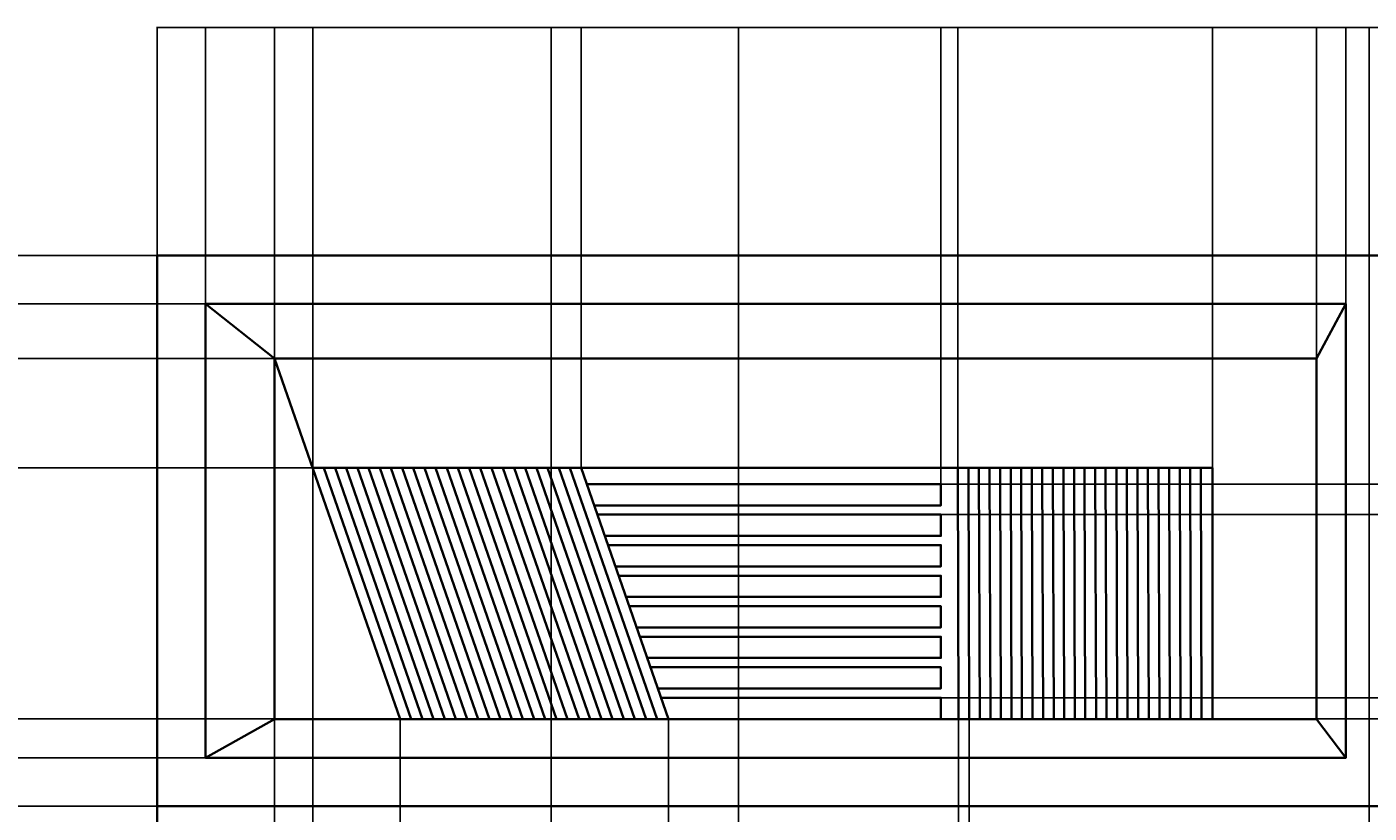
# Model space of a CAD drawing. Units: feet. Extents: x 1141 to 2858, y 751 to 1654.
# Tile 12 of 13: x 2288 to 2610, y 1466 to 1654. Entities that reach past the tile are written whole.
import ezdxf

# ---------------------------------------------------------------- set-up
doc = ezdxf.new("R2010")
doc.units = ezdxf.units.FT
doc.layers.add('A-ANNO-DIMS', color=2, linetype='Continuous', lineweight=18)
doc.layers.add('A-ELEV', color=7, linetype='Continuous', lineweight=35)
doc.styles.get("Standard").update_dxf_attribs({"font": 'arial.ttf'})
doc.dimstyles.get("Standard").update_dxf_attribs({"dimtxt": 0.18, "dimasz": 0.18, "dimexe": 0.18, "dimexo": 0.0625, "dimgap": 0.09, "dimtad": 0, "dimtih": 1, "dimtoh": 1, "dimdec": 1, "dimzin": 0, "dimdsep": 46, "dimlunit": 3, "dimtxsty": 'Standard', "dimcen": 0.09, "dimadec": 0, "dimazin": 0, "dimtfac": 1, "dimtdec": 1, "dimtofl": 0, "dimtmove": 0, "dimatfit": 3, "dimfxl": 1, "dimtolj": 1, "dimtzin": 0, "dimarcsym": 0})

# ---------------------------------------------------------------- blocks, each defined once
blk = doc.blocks.new('*D33')
at = {"layer": 'A-ANNO-DIMS', "color": 0, "lineweight": -2, "transparency": 16777216}
for p, q in [((2117.47, 1467.45), (2857.83, 1467.45)), ((2857.65, 1467.27), (2857.65, 1399.94)), ((2857.65, 1332.24), (2857.65, 1399.58)), ((2117.47, 1332.06), (2857.83, 1332.06))]:
    blk.add_line(p, q, dxfattribs=at)
at = {"layer": 'A-ANNO-DIMS', "color": 0, "transparency": 16777216}
for points in [[(2857.62, 1467.27), (2857.68, 1467.27), (2857.65, 1467.45)], [(2857.62, 1332.24), (2857.68, 1332.24), (2857.65, 1332.06)]]:
    blk.add_solid(points, dxfattribs=at)
at = {"layer": 'Defpoints', "color": 0, "transparency": 16777216}
for p in [(2117.41, 1467.45), (2857.65, 1467.45), (2117.41, 1332.06)]:
    blk.add_point(p, dxfattribs=at)
at = {"layer": 'A-ANNO-DIMS', "color": 0, "transparency": 16777216, "insert": (2857.65, 1399.76), "char_height": 0.18, "attachment_point": 5}
blk.add_mtext('\\A1;135.4', dxfattribs=at)
blk = doc.blocks.new('*D34')
at = {"layer": 'A-ANNO-DIMS', "color": 0, "lineweight": -2, "transparency": 16777216}
for p, q in [((2117.47, 1599.45), (2857.83, 1599.45)), ((2857.65, 1599.27), (2857.65, 1533.63)), ((2857.65, 1467.63), (2857.65, 1533.27)), ((2117.47, 1467.45), (2857.83, 1467.45))]:
    blk.add_line(p, q, dxfattribs=at)
at = {"layer": 'A-ANNO-DIMS', "color": 0, "transparency": 16777216}
for points in [[(2857.62, 1599.27), (2857.68, 1599.27), (2857.65, 1599.45)], [(2857.62, 1467.63), (2857.68, 1467.63), (2857.65, 1467.45)]]:
    blk.add_solid(points, dxfattribs=at)
at = {"layer": 'Defpoints', "color": 0, "transparency": 16777216}
for p in [(2117.41, 1599.45), (2857.65, 1599.45), (2117.41, 1467.45)]:
    blk.add_point(p, dxfattribs=at)
at = {"layer": 'A-ANNO-DIMS', "color": 0, "transparency": 16777216, "insert": (2857.65, 1533.45), "char_height": 0.18, "attachment_point": 5}
blk.add_mtext('\\A1;132', dxfattribs=at)
blk = doc.blocks.new('*D35')
at = {"layer": 'A-ANNO-DIMS', "color": 0, "lineweight": -2, "transparency": 16777216}
for p, q in [((2319.3, 1599.52), (2319.3, 1654.28)), ((2319.48, 1654.1), (2559.01, 1654.1)), ((2799.12, 1654.1), (2559.59, 1654.1)), ((2799.3, 1599.52), (2799.3, 1654.28))]:
    blk.add_line(p, q, dxfattribs=at)
at = {"layer": 'A-ANNO-DIMS', "color": 0, "transparency": 16777216}
for points in [[(2319.48, 1654.13), (2319.48, 1654.07), (2319.3, 1654.1)], [(2799.12, 1654.13), (2799.12, 1654.07), (2799.3, 1654.1)]]:
    blk.add_solid(points, dxfattribs=at)
at = {"layer": 'Defpoints', "color": 0, "transparency": 16777216}
for p in [(2799.3, 1654.1), (2319.3, 1599.45), (2799.3, 1599.45)]:
    blk.add_point(p, dxfattribs=at)
at = {"layer": 'A-ANNO-DIMS', "color": 0, "transparency": 16777216, "insert": (2559.3, 1654.1), "char_height": 0.18, "attachment_point": 5}
blk.add_mtext('\\A1;480', dxfattribs=at)
blk = doc.blocks.new('*D39')
at = {"layer": 'A-ANNO-DIMS', "color": 0, "lineweight": -2, "transparency": 16777216}
for p, q in [((2319.24, 1599.45), (1668.14, 1599.45)), ((1668.32, 1599.27), (1668.32, 1202.86)), ((1668.32, 806.08), (1668.32, 1202.49)), ((2319.24, 805.9), (1668.14, 805.9))]:
    blk.add_line(p, q, dxfattribs=at)
at = {"layer": 'A-ANNO-DIMS', "color": 0, "transparency": 16777216}
for points in [[(1668.29, 1599.27), (1668.35, 1599.27), (1668.32, 1599.45)], [(1668.29, 806.08), (1668.35, 806.08), (1668.32, 805.9)]]:
    blk.add_solid(points, dxfattribs=at)
at = {"layer": 'Defpoints', "color": 0, "transparency": 16777216}
for p in [(1668.32, 1599.45), (2319.3, 1599.45), (2319.3, 805.9)]:
    blk.add_point(p, dxfattribs=at)
at = {"layer": 'A-ANNO-DIMS', "color": 0, "transparency": 16777216, "insert": (1668.32, 1202.68), "char_height": 0.18, "attachment_point": 5}
blk.add_mtext('\\A1;793.6', dxfattribs=at)
blk = doc.blocks.new('*D42')
at = {"layer": 'A-ANNO-DIMS', "color": 0, "lineweight": -2, "transparency": 16777216}
for p, q in [((2319.3, 1599.52), (2319.3, 1654.28)), ((2319.48, 1654.1), (2324.71, 1654.1)), ((2330.7, 1654.1), (2325.48, 1654.1)), ((2330.88, 1587.93), (2330.88, 1654.28))]:
    blk.add_line(p, q, dxfattribs=at)
at = {"layer": 'A-ANNO-DIMS', "color": 0, "transparency": 16777216}
for points in [[(2319.48, 1654.13), (2319.48, 1654.07), (2319.3, 1654.1)], [(2330.7, 1654.13), (2330.7, 1654.07), (2330.88, 1654.1)]]:
    blk.add_solid(points, dxfattribs=at)
at = {"layer": 'Defpoints', "color": 0, "transparency": 16777216}
for p in [(2330.88, 1654.1), (2319.3, 1599.45), (2330.88, 1587.87)]:
    blk.add_point(p, dxfattribs=at)
at = {"layer": 'A-ANNO-DIMS', "color": 0, "transparency": 16777216, "insert": (2325.09, 1654.1), "char_height": 0.18, "attachment_point": 5}
blk.add_mtext('\\A1;11.58', dxfattribs=at)
blk = doc.blocks.new('*D43')
at = {"layer": 'A-ANNO-DIMS', "color": 0, "lineweight": -2, "transparency": 16777216}
for p, q in [((2330.88, 1587.93), (2330.88, 1654.28)), ((2331.06, 1654.1), (2338.81, 1654.1)), ((2347.33, 1654.1), (2339.58, 1654.1)), ((2347.51, 1574.83), (2347.51, 1654.28))]:
    blk.add_line(p, q, dxfattribs=at)
at = {"layer": 'A-ANNO-DIMS', "color": 0, "transparency": 16777216}
for points in [[(2331.06, 1654.13), (2331.06, 1654.07), (2330.88, 1654.1)], [(2347.33, 1654.13), (2347.33, 1654.07), (2347.51, 1654.1)]]:
    blk.add_solid(points, dxfattribs=at)
at = {"layer": 'Defpoints', "color": 0, "transparency": 16777216}
for p in [(2347.51, 1654.1), (2330.88, 1587.87), (2347.51, 1574.77)]:
    blk.add_point(p, dxfattribs=at)
at = {"layer": 'A-ANNO-DIMS', "color": 0, "transparency": 16777216, "insert": (2339.2, 1654.1), "char_height": 0.18, "attachment_point": 5}
blk.add_mtext('\\A1;16.63', dxfattribs=at)
blk = doc.blocks.new('*D44')
at = {"layer": 'A-ANNO-DIMS', "color": 0, "lineweight": -2, "transparency": 16777216}
for p, q in [((2347.51, 1574.83), (2347.51, 1654.28)), ((2347.69, 1654.1), (2472.22, 1654.1)), ((2597.32, 1654.1), (2472.8, 1654.1)), ((2597.5, 1574.83), (2597.5, 1654.28))]:
    blk.add_line(p, q, dxfattribs=at)
at = {"layer": 'A-ANNO-DIMS', "color": 0, "transparency": 16777216}
for points in [[(2347.69, 1654.13), (2347.69, 1654.07), (2347.51, 1654.1)], [(2597.32, 1654.13), (2597.32, 1654.07), (2597.5, 1654.1)]]:
    blk.add_solid(points, dxfattribs=at)
at = {"layer": 'Defpoints', "color": 0, "transparency": 16777216}
for p in [(2597.5, 1654.1), (2347.51, 1574.77), (2597.5, 1574.77)]:
    blk.add_point(p, dxfattribs=at)
at = {"layer": 'A-ANNO-DIMS', "color": 0, "transparency": 16777216, "insert": (2472.51, 1654.1), "char_height": 0.18, "attachment_point": 5}
blk.add_mtext('\\A1;250', dxfattribs=at)
blk = doc.blocks.new('*D45')
at = {"layer": 'A-ANNO-DIMS', "color": 0, "lineweight": -2, "transparency": 16777216}
for p, q in [((2597.5, 1574.83), (2597.5, 1654.28)), ((2597.68, 1654.1), (2600.64, 1654.1)), ((2604.38, 1654.1), (2601.42, 1654.1)), ((2604.56, 1587.93), (2604.56, 1654.28))]:
    blk.add_line(p, q, dxfattribs=at)
at = {"layer": 'A-ANNO-DIMS', "color": 0, "transparency": 16777216}
for points in [[(2597.68, 1654.13), (2597.68, 1654.07), (2597.5, 1654.1)], [(2604.38, 1654.13), (2604.38, 1654.07), (2604.56, 1654.1)]]:
    blk.add_solid(points, dxfattribs=at)
at = {"layer": 'Defpoints', "color": 0, "transparency": 16777216}
for p in [(2604.56, 1654.1), (2604.56, 1587.87), (2597.5, 1574.77)]:
    blk.add_point(p, dxfattribs=at)
at = {"layer": 'A-ANNO-DIMS', "color": 0, "transparency": 16777216, "insert": (2601.03, 1654.1), "char_height": 0.18, "attachment_point": 5}
blk.add_mtext('\\A1;7.054', dxfattribs=at)
blk = doc.blocks.new('*D46')
at = {"layer": 'A-ANNO-DIMS', "color": 0, "lineweight": -2, "transparency": 16777216}
for p, q in [((2604.56, 1587.93), (2604.56, 1654.28)), ((2604.74, 1654.1), (2609.96, 1654.1)), ((2615.96, 1654.1), (2610.73, 1654.1)), ((2616.14, 1599.52), (2616.14, 1654.28))]:
    blk.add_line(p, q, dxfattribs=at)
at = {"layer": 'A-ANNO-DIMS', "color": 0, "transparency": 16777216}
for points in [[(2604.74, 1654.13), (2604.74, 1654.07), (2604.56, 1654.1)], [(2615.96, 1654.13), (2615.96, 1654.07), (2616.14, 1654.1)]]:
    blk.add_solid(points, dxfattribs=at)
at = {"layer": 'Defpoints', "color": 0, "transparency": 16777216}
for p in [(2616.14, 1654.1), (2616.14, 1599.45), (2604.56, 1587.87)]:
    blk.add_point(p, dxfattribs=at)
at = {"layer": 'A-ANNO-DIMS', "color": 0, "transparency": 16777216, "insert": (2610.35, 1654.1), "char_height": 0.18, "attachment_point": 5}
blk.add_mtext('\\A1;11.58', dxfattribs=at)
blk = doc.blocks.new('*D48')
at = {"layer": 'A-ANNO-DIMS', "color": 0, "lineweight": -2, "transparency": 16777216}
for p, q in [((2330.82, 1479.03), (1668.14, 1479.03)), ((1668.32, 1478.85), (1668.32, 1473.42)), ((1668.32, 1467.63), (1668.32, 1473.06)), ((2319.24, 1467.45), (1668.14, 1467.45))]:
    blk.add_line(p, q, dxfattribs=at)
at = {"layer": 'A-ANNO-DIMS', "color": 0, "transparency": 16777216}
for points in [[(1668.29, 1478.85), (1668.35, 1478.85), (1668.32, 1479.03)], [(1668.29, 1467.63), (1668.35, 1467.63), (1668.32, 1467.45)]]:
    blk.add_solid(points, dxfattribs=at)
at = {"layer": 'Defpoints', "color": 0, "transparency": 16777216}
for p in [(1668.32, 1479.03), (2330.88, 1479.03), (2319.3, 1467.45)]:
    blk.add_point(p, dxfattribs=at)
at = {"layer": 'A-ANNO-DIMS', "color": 0, "transparency": 16777216, "insert": (1668.32, 1473.24), "char_height": 0.18, "attachment_point": 5}
blk.add_mtext('\\A1;11.58', dxfattribs=at)
blk = doc.blocks.new('*D49')
at = {"layer": 'A-ANNO-DIMS', "color": 0, "lineweight": -2, "transparency": 16777216}
for p, q in [((2347.45, 1488.33), (1668.14, 1488.33)), ((1668.32, 1488.15), (1668.32, 1483.86)), ((1668.32, 1479.21), (1668.32, 1483.5)), ((2330.82, 1479.03), (1668.14, 1479.03))]:
    blk.add_line(p, q, dxfattribs=at)
at = {"layer": 'A-ANNO-DIMS', "color": 0, "transparency": 16777216}
for points in [[(1668.29, 1488.15), (1668.35, 1488.15), (1668.32, 1488.33)], [(1668.29, 1479.21), (1668.35, 1479.21), (1668.32, 1479.03)]]:
    blk.add_solid(points, dxfattribs=at)
at = {"layer": 'Defpoints', "color": 0, "transparency": 16777216}
for p in [(1668.32, 1488.33), (2347.51, 1488.33), (2330.88, 1479.03)]:
    blk.add_point(p, dxfattribs=at)
at = {"layer": 'A-ANNO-DIMS', "color": 0, "transparency": 16777216, "insert": (1668.32, 1483.68), "char_height": 0.18, "attachment_point": 5}
blk.add_mtext('\\A1;9.293', dxfattribs=at)
blk = doc.blocks.new('*D50')
at = {"layer": 'A-ANNO-DIMS', "color": 0, "lineweight": -2, "transparency": 16777216}
for p, q in [((2356.58, 1548.54), (1668.14, 1548.54)), ((1668.32, 1548.36), (1668.32, 1518.62)), ((1668.32, 1488.51), (1668.32, 1518.25)), ((2347.45, 1488.33), (1668.14, 1488.33))]:
    blk.add_line(p, q, dxfattribs=at)
at = {"layer": 'A-ANNO-DIMS', "color": 0, "transparency": 16777216}
for points in [[(1668.29, 1548.36), (1668.35, 1548.36), (1668.32, 1548.54)], [(1668.29, 1488.51), (1668.35, 1488.51), (1668.32, 1488.33)]]:
    blk.add_solid(points, dxfattribs=at)
at = {"layer": 'Defpoints', "color": 0, "transparency": 16777216}
for p in [(1668.32, 1548.54), (2356.64, 1548.54), (2347.51, 1488.33)]:
    blk.add_point(p, dxfattribs=at)
at = {"layer": 'A-ANNO-DIMS', "color": 0, "transparency": 16777216, "insert": (1668.32, 1518.43), "char_height": 0.18, "attachment_point": 5}
blk.add_mtext('\\A1;60.22', dxfattribs=at)
blk = doc.blocks.new('*D51')
at = {"layer": 'A-ANNO-DIMS', "color": 0, "lineweight": -2, "transparency": 16777216}
for p, q in [((2347.45, 1574.77), (1668.14, 1574.77)), ((1668.32, 1574.59), (1668.32, 1561.84)), ((1668.32, 1548.72), (1668.32, 1561.47)), ((2356.58, 1548.54), (1668.14, 1548.54))]:
    blk.add_line(p, q, dxfattribs=at)
at = {"layer": 'A-ANNO-DIMS', "color": 0, "transparency": 16777216}
for points in [[(1668.29, 1574.59), (1668.35, 1574.59), (1668.32, 1574.77)], [(1668.29, 1548.72), (1668.35, 1548.72), (1668.32, 1548.54)]]:
    blk.add_solid(points, dxfattribs=at)
at = {"layer": 'Defpoints', "color": 0, "transparency": 16777216}
for p in [(1668.32, 1574.77), (2347.51, 1574.77), (2356.64, 1548.54)]:
    blk.add_point(p, dxfattribs=at)
at = {"layer": 'A-ANNO-DIMS', "color": 0, "transparency": 16777216, "insert": (1668.32, 1561.66), "char_height": 0.18, "attachment_point": 5}
blk.add_mtext('\\A1;26.23', dxfattribs=at)
blk = doc.blocks.new('*D52')
at = {"layer": 'A-ANNO-DIMS', "color": 0, "lineweight": -2, "transparency": 16777216}
for p, q in [((2330.82, 1587.87), (1668.14, 1587.87)), ((1668.32, 1587.69), (1668.32, 1581.5)), ((1668.32, 1574.95), (1668.32, 1581.14)), ((2347.45, 1574.77), (1668.14, 1574.77))]:
    blk.add_line(p, q, dxfattribs=at)
at = {"layer": 'A-ANNO-DIMS', "color": 0, "transparency": 16777216}
for points in [[(1668.29, 1587.69), (1668.35, 1587.69), (1668.32, 1587.87)], [(1668.29, 1574.95), (1668.35, 1574.95), (1668.32, 1574.77)]]:
    blk.add_solid(points, dxfattribs=at)
at = {"layer": 'Defpoints', "color": 0, "transparency": 16777216}
for p in [(1668.32, 1587.87), (2330.88, 1587.87), (2347.51, 1574.77)]:
    blk.add_point(p, dxfattribs=at)
at = {"layer": 'A-ANNO-DIMS', "color": 0, "transparency": 16777216, "insert": (1668.32, 1581.32), "char_height": 0.18, "attachment_point": 5}
blk.add_mtext('\\A1;13.102', dxfattribs=at)
blk = doc.blocks.new('*D53')
at = {"layer": 'A-ANNO-DIMS', "color": 0, "lineweight": -2, "transparency": 16777216}
for p, q in [((2319.24, 1599.45), (1668.14, 1599.45)), ((1668.32, 1599.27), (1668.32, 1593.84)), ((1668.32, 1588.05), (1668.32, 1593.48)), ((2330.82, 1587.87), (1668.14, 1587.87))]:
    blk.add_line(p, q, dxfattribs=at)
at = {"layer": 'A-ANNO-DIMS', "color": 0, "transparency": 16777216}
for points in [[(1668.29, 1599.27), (1668.35, 1599.27), (1668.32, 1599.45)], [(1668.29, 1588.05), (1668.35, 1588.05), (1668.32, 1587.87)]]:
    blk.add_solid(points, dxfattribs=at)
at = {"layer": 'Defpoints', "color": 0, "transparency": 16777216}
for p in [(1668.32, 1599.45), (2319.3, 1599.45), (2330.88, 1587.87)]:
    blk.add_point(p, dxfattribs=at)
at = {"layer": 'A-ANNO-DIMS', "color": 0, "transparency": 16777216, "insert": (1668.32, 1593.66), "char_height": 0.18, "attachment_point": 5}
blk.add_mtext('\\A1;11.58', dxfattribs=at)
blk = doc.blocks.new('*D55')
at = {"layer": 'A-ANNO-DIMS', "color": 0, "lineweight": -2, "transparency": 16777216}
for p, q in [((2347.51, 1574.71), (2347.51, 751.07)), ((2356.64, 1548.48), (2356.64, 751.07)), ((2347.69, 751.25), (2351.75, 751.25)), ((2356.46, 751.25), (2352.4, 751.25))]:
    blk.add_line(p, q, dxfattribs=at)
at = {"layer": 'A-ANNO-DIMS', "color": 0, "transparency": 16777216}
for points in [[(2347.69, 751.28), (2347.69, 751.22), (2347.51, 751.25)], [(2356.46, 751.28), (2356.46, 751.22), (2356.64, 751.25)]]:
    blk.add_solid(points, dxfattribs=at)
at = {"layer": 'Defpoints', "color": 0, "transparency": 16777216}
for p in [(2347.51, 1574.77), (2356.64, 1548.54), (2356.64, 751.25)]:
    blk.add_point(p, dxfattribs=at)
at = {"layer": 'A-ANNO-DIMS', "color": 0, "transparency": 16777216, "insert": (2352.08, 751.25), "char_height": 0.18, "attachment_point": 5}
blk.add_mtext('\\A1;9.13', dxfattribs=at)
blk = doc.blocks.new('*D56')
at = {"layer": 'A-ANNO-DIMS', "color": 0, "lineweight": -2, "transparency": 16777216}
for p, q in [((2356.64, 1548.6), (2356.64, 1654.28)), ((2356.82, 1654.1), (2388.52, 1654.1)), ((2420.87, 1654.1), (2389.17, 1654.1)), ((2421.05, 1548.6), (2421.05, 1654.28))]:
    blk.add_line(p, q, dxfattribs=at)
at = {"layer": 'A-ANNO-DIMS', "color": 0, "transparency": 16777216}
for points in [[(2356.82, 1654.13), (2356.82, 1654.07), (2356.64, 1654.1)], [(2420.87, 1654.13), (2420.87, 1654.07), (2421.05, 1654.1)]]:
    blk.add_solid(points, dxfattribs=at)
at = {"layer": 'Defpoints', "color": 0, "transparency": 16777216}
for p in [(2421.05, 1654.1), (2356.64, 1548.54), (2421.05, 1548.54)]:
    blk.add_point(p, dxfattribs=at)
at = {"layer": 'A-ANNO-DIMS', "color": 0, "transparency": 16777216, "insert": (2388.85, 1654.1), "char_height": 0.18, "attachment_point": 5}
blk.add_mtext('\\A1;64.4', dxfattribs=at)
blk = doc.blocks.new('*D57')
at = {"layer": 'A-ANNO-DIMS', "color": 0, "lineweight": -2, "transparency": 16777216}
for p, q in [((2421.05, 1548.6), (2421.05, 1654.28)), ((2421.23, 1654.1), (2463.82, 1654.1)), ((2507.21, 1654.1), (2464.61, 1654.1)), ((2507.39, 1544.71), (2507.39, 1654.28))]:
    blk.add_line(p, q, dxfattribs=at)
at = {"layer": 'A-ANNO-DIMS', "color": 0, "transparency": 16777216}
for points in [[(2421.23, 1654.13), (2421.23, 1654.07), (2421.05, 1654.1)], [(2507.21, 1654.13), (2507.21, 1654.07), (2507.39, 1654.1)]]:
    blk.add_solid(points, dxfattribs=at)
at = {"layer": 'Defpoints', "color": 0, "transparency": 16777216}
for p in [(2507.39, 1654.1), (2421.05, 1548.54), (2507.39, 1544.65)]:
    blk.add_point(p, dxfattribs=at)
at = {"layer": 'A-ANNO-DIMS', "color": 0, "transparency": 16777216, "insert": (2464.22, 1654.1), "char_height": 0.18, "attachment_point": 5}
blk.add_mtext('\\A1;86.34', dxfattribs=at)
blk = doc.blocks.new('*D58')
at = {"layer": 'A-ANNO-DIMS', "color": 0, "lineweight": -2, "transparency": 16777216}
for p, q in [((2507.39, 1544.71), (2507.39, 1654.28)), ((2507.57, 1654.1), (2509.01, 1654.1)), ((2511.25, 1654.1), (2509.81, 1654.1)), ((2511.43, 1548.6), (2511.43, 1654.28))]:
    blk.add_line(p, q, dxfattribs=at)
at = {"layer": 'A-ANNO-DIMS', "color": 0, "transparency": 16777216}
for points in [[(2507.57, 1654.13), (2507.57, 1654.07), (2507.39, 1654.1)], [(2511.25, 1654.13), (2511.25, 1654.07), (2511.43, 1654.1)]]:
    blk.add_solid(points, dxfattribs=at)
at = {"layer": 'Defpoints', "color": 0, "transparency": 16777216}
for p in [(2511.43, 1654.1), (2511.43, 1548.54), (2507.39, 1544.65)]:
    blk.add_point(p, dxfattribs=at)
at = {"layer": 'A-ANNO-DIMS', "color": 0, "transparency": 16777216, "insert": (2509.41, 1654.1), "char_height": 0.18, "attachment_point": 5}
blk.add_mtext('\\A1;4.045', dxfattribs=at)
blk = doc.blocks.new('*D59')
at = {"layer": 'A-ANNO-DIMS', "color": 0, "lineweight": -2, "transparency": 16777216}
for p, q in [((2511.43, 1548.6), (2511.43, 1654.28)), ((2511.61, 1654.1), (2541.58, 1654.1)), ((2572.34, 1654.1), (2542.37, 1654.1)), ((2572.52, 1548.6), (2572.52, 1654.28))]:
    blk.add_line(p, q, dxfattribs=at)
at = {"layer": 'A-ANNO-DIMS', "color": 0, "transparency": 16777216}
for points in [[(2511.61, 1654.13), (2511.61, 1654.07), (2511.43, 1654.1)], [(2572.34, 1654.13), (2572.34, 1654.07), (2572.52, 1654.1)]]:
    blk.add_solid(points, dxfattribs=at)
at = {"layer": 'Defpoints', "color": 0, "transparency": 16777216}
for p in [(2572.52, 1654.1), (2511.43, 1548.54), (2572.52, 1548.54)]:
    blk.add_point(p, dxfattribs=at)
at = {"layer": 'A-ANNO-DIMS', "color": 0, "transparency": 16777216, "insert": (2541.97, 1654.1), "char_height": 0.18, "attachment_point": 5}
blk.add_mtext('\\A1;61.09', dxfattribs=at)
blk = doc.blocks.new('*D60')
at = {"layer": 'A-ANNO-DIMS', "color": 0, "lineweight": -2, "transparency": 16777216}
for p, q in [((2572.52, 1548.6), (2572.52, 1654.28)), ((2572.7, 1654.1), (2584.54, 1654.1)), ((2597.32, 1654.1), (2585.48, 1654.1)), ((2597.5, 1574.83), (2597.5, 1654.28))]:
    blk.add_line(p, q, dxfattribs=at)
at = {"layer": 'A-ANNO-DIMS', "color": 0, "transparency": 16777216}
for points in [[(2572.7, 1654.13), (2572.7, 1654.07), (2572.52, 1654.1)], [(2597.32, 1654.13), (2597.32, 1654.07), (2597.5, 1654.1)]]:
    blk.add_solid(points, dxfattribs=at)
at = {"layer": 'Defpoints', "color": 0, "transparency": 16777216}
for p in [(2597.5, 1654.1), (2597.5, 1574.77), (2572.52, 1548.54)]:
    blk.add_point(p, dxfattribs=at)
at = {"layer": 'A-ANNO-DIMS', "color": 0, "transparency": 16777216, "insert": (2585.01, 1654.1), "char_height": 0.18, "attachment_point": 5}
blk.add_mtext('\\A1;24.983', dxfattribs=at)
blk = doc.blocks.new('*D61')
at = {"layer": 'A-ANNO-DIMS', "color": 0, "lineweight": -2, "transparency": 16777216}
for p, q in [((2347.51, 1488.26), (2347.51, 751.07)), ((2377.6, 1488.26), (2377.6, 751.07)), ((2347.69, 751.25), (2362.16, 751.25)), ((2377.42, 751.25), (2362.95, 751.25))]:
    blk.add_line(p, q, dxfattribs=at)
at = {"layer": 'A-ANNO-DIMS', "color": 0, "transparency": 16777216}
for points in [[(2347.69, 751.28), (2347.69, 751.22), (2347.51, 751.25)], [(2377.42, 751.28), (2377.42, 751.22), (2377.6, 751.25)]]:
    blk.add_solid(points, dxfattribs=at)
at = {"layer": 'Defpoints', "color": 0, "transparency": 16777216}
for p in [(2347.51, 1488.33), (2377.6, 1488.33), (2377.6, 751.25)]:
    blk.add_point(p, dxfattribs=at)
at = {"layer": 'A-ANNO-DIMS', "color": 0, "transparency": 16777216, "insert": (2362.56, 751.25), "char_height": 0.18, "attachment_point": 5}
blk.add_mtext('\\A1;30.09', dxfattribs=at)
blk = doc.blocks.new('*D62')
at = {"layer": 'A-ANNO-DIMS', "color": 0, "lineweight": -2, "transparency": 16777216}
for p, q in [((2377.6, 1488.26), (2377.6, 751.07)), ((2442.01, 1488.26), (2442.01, 751.07)), ((2377.78, 751.25), (2409.48, 751.25)), ((2441.83, 751.25), (2410.13, 751.25))]:
    blk.add_line(p, q, dxfattribs=at)
at = {"layer": 'A-ANNO-DIMS', "color": 0, "transparency": 16777216}
for points in [[(2377.78, 751.28), (2377.78, 751.22), (2377.6, 751.25)], [(2441.83, 751.28), (2441.83, 751.22), (2442.01, 751.25)]]:
    blk.add_solid(points, dxfattribs=at)
at = {"layer": 'Defpoints', "color": 0, "transparency": 16777216}
for p in [(2377.6, 1488.33), (2442.01, 1488.33), (2442.01, 751.25)]:
    blk.add_point(p, dxfattribs=at)
at = {"layer": 'A-ANNO-DIMS', "color": 0, "transparency": 16777216, "insert": (2409.81, 751.25), "char_height": 0.18, "attachment_point": 5}
blk.add_mtext('\\A1;64.4', dxfattribs=at)
blk = doc.blocks.new('*D63')
at = {"layer": 'A-ANNO-DIMS', "color": 0, "lineweight": -2, "transparency": 16777216}
for p, q in [((2511.62, 1488.26), (2511.62, 751.07)), ((2514.19, 1488.26), (2514.19, 751.07)), ((2511.8, 751.25), (2512.58, 751.25)), ((2514.01, 751.25), (2513.23, 751.25))]:
    blk.add_line(p, q, dxfattribs=at)
at = {"layer": 'A-ANNO-DIMS', "color": 0, "transparency": 16777216}
for points in [[(2511.8, 751.28), (2511.8, 751.22), (2511.62, 751.25)], [(2514.01, 751.28), (2514.01, 751.22), (2514.19, 751.25)]]:
    blk.add_solid(points, dxfattribs=at)
at = {"layer": 'Defpoints', "color": 0, "transparency": 16777216}
for p in [(2511.62, 1488.33), (2514.19, 1488.33), (2514.19, 751.25)]:
    blk.add_point(p, dxfattribs=at)
at = {"layer": 'A-ANNO-DIMS', "color": 0, "transparency": 16777216, "insert": (2512.91, 751.25), "char_height": 0.18, "attachment_point": 5}
blk.add_mtext('\\A1;2.57', dxfattribs=at)
blk = doc.blocks.new('*D64')
at = {"layer": 'A-ANNO-DIMS', "color": 0, "lineweight": -2, "transparency": 16777216}
for p, q in [((2507.45, 1544.65), (2857.83, 1544.65)), ((2857.65, 1544.47), (2857.65, 1541.17)), ((2857.65, 1537.51), (2857.65, 1540.81)), ((2507.45, 1537.33), (2857.83, 1537.33))]:
    blk.add_line(p, q, dxfattribs=at)
at = {"layer": 'A-ANNO-DIMS', "color": 0, "transparency": 16777216}
for points in [[(2857.62, 1544.47), (2857.68, 1544.47), (2857.65, 1544.65)], [(2857.62, 1537.51), (2857.68, 1537.51), (2857.65, 1537.33)]]:
    blk.add_solid(points, dxfattribs=at)
at = {"layer": 'Defpoints', "color": 0, "transparency": 16777216}
for p in [(2507.39, 1544.65), (2507.39, 1537.33), (2857.65, 1537.33)]:
    blk.add_point(p, dxfattribs=at)
at = {"layer": 'A-ANNO-DIMS', "color": 0, "transparency": 16777216, "insert": (2857.65, 1540.99), "char_height": 0.18, "attachment_point": 5}
blk.add_mtext('\\A1;7.317', dxfattribs=at)
blk = doc.blocks.new('*D65')
at = {"layer": 'A-ANNO-DIMS', "color": 0, "lineweight": -2, "transparency": 16777216}
for p, q in [((2507.45, 1493.43), (2857.83, 1493.43)), ((2857.65, 1493.25), (2857.65, 1491.06)), ((2507.45, 1488.33), (2857.83, 1488.33)), ((2857.65, 1488.51), (2857.65, 1490.69))]:
    blk.add_line(p, q, dxfattribs=at)
at = {"layer": 'A-ANNO-DIMS', "color": 0, "transparency": 16777216}
for points in [[(2857.62, 1493.25), (2857.68, 1493.25), (2857.65, 1493.43)], [(2857.62, 1488.51), (2857.68, 1488.51), (2857.65, 1488.33)]]:
    blk.add_solid(points, dxfattribs=at)
at = {"layer": 'Defpoints', "color": 0, "transparency": 16777216}
for p in [(2507.39, 1493.43), (2507.39, 1488.33), (2857.65, 1488.33)]:
    blk.add_point(p, dxfattribs=at)
at = {"layer": 'A-ANNO-DIMS', "color": 0, "transparency": 16777216, "insert": (2857.65, 1490.88), "char_height": 0.18, "attachment_point": 5}
blk.add_mtext('\\A1;5.099', dxfattribs=at)
blk = doc.blocks.new('*D82')
at = {"layer": 'A-ANNO-DIMS', "color": 0, "lineweight": -2, "transparency": 16777216}
for p, q in [((2319.3, 1196.74), (2319.3, 1654.28)), ((2319.48, 1654.1), (2388.58, 1654.1)), ((2458.6, 1654.1), (2389.49, 1654.1)), ((2458.78, 1222.3), (2458.78, 1654.28))]:
    blk.add_line(p, q, dxfattribs=at)
at = {"layer": 'A-ANNO-DIMS', "color": 0, "transparency": 16777216}
for points in [[(2319.48, 1654.13), (2319.48, 1654.07), (2319.3, 1654.1)], [(2458.6, 1654.13), (2458.6, 1654.07), (2458.78, 1654.1)]]:
    blk.add_solid(points, dxfattribs=at)
at = {"layer": 'Defpoints', "color": 0, "transparency": 16777216}
for p in [(2458.78, 1654.1), (2458.78, 1222.24), (2319.3, 1196.68)]:
    blk.add_point(p, dxfattribs=at)
at = {"layer": 'A-ANNO-DIMS', "color": 0, "transparency": 16777216, "insert": (2389.04, 1654.1), "char_height": 0.18, "attachment_point": 5}
blk.add_mtext('\\A1;139.47', dxfattribs=at)
blk = doc.blocks.new('*D83')
at = {"layer": 'A-ANNO-DIMS', "color": 0, "lineweight": -2, "transparency": 16777216}
for p, q in [((2319.3, 1196.74), (2319.3, 1654.28)), ((2319.48, 1654.1), (2464.26, 1654.1)), ((2609.96, 1654.1), (2465.19, 1654.1)), ((2610.14, 1217.61), (2610.14, 1654.28))]:
    blk.add_line(p, q, dxfattribs=at)
at = {"layer": 'A-ANNO-DIMS', "color": 0, "transparency": 16777216}
for points in [[(2319.48, 1654.13), (2319.48, 1654.07), (2319.3, 1654.1)], [(2609.96, 1654.13), (2609.96, 1654.07), (2610.14, 1654.1)]]:
    blk.add_solid(points, dxfattribs=at)
at = {"layer": 'Defpoints', "color": 0, "transparency": 16777216}
for p in [(2610.14, 1654.1), (2610.14, 1217.55), (2319.3, 1196.68)]:
    blk.add_point(p, dxfattribs=at)
at = {"layer": 'A-ANNO-DIMS', "color": 0, "transparency": 16777216, "insert": (2464.72, 1654.1), "char_height": 0.18, "attachment_point": 5}
blk.add_mtext('\\A1;290.84', dxfattribs=at)
blk = doc.blocks.new('*D86')
at = {"layer": 'A-ANNO-DIMS', "color": 0, "lineweight": -2, "transparency": 16777216}
for p, q in [((2413.84, 1332.13), (2413.84, 1654.28)), ((2414.02, 1654.1), (2435.91, 1654.1)), ((2458.6, 1654.1), (2436.71, 1654.1)), ((2458.78, 1357.69), (2458.78, 1654.28))]:
    blk.add_line(p, q, dxfattribs=at)
at = {"layer": 'A-ANNO-DIMS', "color": 0, "transparency": 16777216}
for points in [[(2414.02, 1654.13), (2414.02, 1654.07), (2413.84, 1654.1)], [(2458.6, 1654.13), (2458.6, 1654.07), (2458.78, 1654.1)]]:
    blk.add_solid(points, dxfattribs=at)
at = {"layer": 'Defpoints', "color": 0, "transparency": 16777216}
for p in [(2458.78, 1654.1), (2458.78, 1357.62), (2413.84, 1332.06)]:
    blk.add_point(p, dxfattribs=at)
at = {"layer": 'A-ANNO-DIMS', "color": 0, "transparency": 16777216, "insert": (2436.31, 1654.1), "char_height": 0.18, "attachment_point": 5}
blk.add_mtext('\\A1;44.93', dxfattribs=at)

msp = doc.modelspace()

# ---------------------------------------------------------------- linework, layer by layer
at = {"layer": 'A-ELEV'}
for p, q in [((2319.3013, 1599.4527), (2319.3013, 919.339)), ((2330.8815, 1587.8725), (2347.5116, 1574.7702)), ((2597.5015, 1574.7702), (2604.5555, 1587.8725)), ((2347.5116, 1574.7702), (2347.5116, 1488.3255)), ((2347.5116, 1574.7702), (2597.5015, 1574.7702)), ((2347.5116, 1574.7702), (2377.6041, 1488.3255)), ((2597.5015, 1574.7702), (2597.5015, 1488.2273)), ((2356.6424, 1548.5407), (2572.5184, 1548.5407)), ((2572.5184, 1548.5407), (2572.5184, 1488.3255)), ((2347.5116, 1488.3255), (2330.8815, 1479.033)), ((2347.5116, 1488.3255), (2597.5015, 1488.3255)), ((2597.5015, 1488.3255), (2604.5555, 1479.033))]:
    msp.add_line(p, q, dxfattribs=at)
for points in [[(2319.3013, 1599.4527), (2616.1358, 1599.4527), (2616.1358, 1467.4527), (2319.3013, 1467.4527)], [(2330.8815, 1587.8725), (2604.5555, 1587.8725), (2604.5555, 1479.033), (2330.8815, 1479.033)]]:
    msp.add_lwpolyline(points, close=True, dxfattribs=at)
for points in [[(2359.2875, 1548.5407), (2380.2492, 1488.3255)], [(2382.9713, 1488.3255), (2362.0095, 1548.5407)], [(2364.6546, 1548.5407), (2385.6163, 1488.3255)], [(2388.3384, 1488.3255), (2367.3767, 1548.5407)], [(2370.0217, 1548.5407), (2390.9835, 1488.3255)], [(2393.7055, 1488.3255), (2372.7438, 1548.5407)], [(2375.3889, 1548.5407), (2396.3506, 1488.3255)], [(2399.0726, 1488.3255), (2378.1109, 1548.5407)], [(2380.756, 1548.5407), (2401.7177, 1488.3255)], [(2404.4397, 1488.3255), (2383.478, 1548.5407)], [(2386.1231, 1548.5407), (2407.0848, 1488.3255)], [(2409.8069, 1488.3255), (2388.8451, 1548.5407)], [(2391.4902, 1548.5407), (2412.4519, 1488.3255)], [(2415.174, 1488.3255), (2394.2123, 1548.5407)], [(2396.8574, 1548.5407), (2417.8191, 1488.3255)], [(2420.5411, 1488.3255), (2399.5794, 1548.5407)], [(2402.2245, 1548.5407), (2423.1862, 1488.3255)], [(2425.9082, 1488.3255), (2404.9465, 1548.5407)], [(2407.5916, 1548.5407), (2428.5533, 1488.3255)], [(2431.2753, 1488.3255), (2410.3136, 1548.5407)], [(2412.9587, 1548.5407), (2433.9204, 1488.3255)], [(2436.6425, 1488.3255), (2415.6808, 1548.5407)], [(2418.3258, 1548.5407), (2439.2876, 1488.3255)], [(2442.0096, 1488.3255), (2421.0479, 1548.5407)], [(2511.4316, 1548.5407), (2511.6201, 1488.3255)], [(2514.1908, 1488.3255), (2514.0024, 1548.5407)], [(2516.5004, 1548.5407), (2516.6889, 1488.3255)], [(2519.2596, 1488.3255), (2519.0712, 1548.5407)], [(2521.5692, 1548.5407), (2521.7577, 1488.3255)], [(2524.3284, 1488.3255), (2524.14, 1548.5407)], [(2526.638, 1548.5407), (2526.8265, 1488.3255)], [(2529.3972, 1488.3255), (2529.2088, 1548.5407)], [(2531.7068, 1548.5407), (2531.8953, 1488.3255)], [(2534.466, 1488.3255), (2534.2776, 1548.5407)], [(2536.7756, 1548.5407), (2536.9641, 1488.3255)], [(2539.5348, 1488.3255), (2539.3464, 1548.5407)], [(2541.8444, 1548.5407), (2542.0329, 1488.3255)], [(2544.6036, 1488.3255), (2544.4152, 1548.5407)], [(2546.9132, 1548.5407), (2547.1017, 1488.3255)], [(2549.6724, 1488.3255), (2549.484, 1548.5407)], [(2551.982, 1548.5407), (2552.1705, 1488.3255)], [(2554.7412, 1488.3255), (2554.5528, 1548.5407)], [(2557.0508, 1548.5407), (2557.2393, 1488.3255)], [(2559.81, 1488.3255), (2559.6216, 1548.5407)], [(2562.1196, 1548.5407), (2562.3081, 1488.3255)], [(2564.8788, 1488.3255), (2564.6904, 1548.5407)], [(2567.1884, 1548.5407), (2567.3769, 1488.3255)], [(2569.9476, 1488.3255), (2569.7592, 1548.5407)], [(2422.4037, 1544.6458), (2507.3869, 1544.6458), (2507.3869, 1539.5463), (2424.1789, 1539.5463)], [(2424.951, 1537.3285), (2507.3869, 1537.3285), (2507.3869, 1532.2291), (2426.7262, 1532.2291)], [(2427.4982, 1530.0113), (2507.3869, 1530.0113), (2507.3869, 1524.9118), (2429.2734, 1524.9118)], [(2430.0454, 1522.694), (2507.3869, 1522.694), (2507.3869, 1517.5946), (2431.8206, 1517.5946)], [(2432.5927, 1515.3768), (2507.3869, 1515.3768), (2507.3869, 1510.2773), (2434.3679, 1510.2773)], [(2435.1399, 1508.0595), (2507.3869, 1508.0595), (2507.3869, 1502.9601), (2436.9151, 1502.9601)], [(2437.6872, 1500.7423), (2507.3869, 1500.7423), (2507.3869, 1495.6428), (2439.4623, 1495.6428)], [(2440.2344, 1493.425), (2507.3869, 1493.425), (2507.3869, 1488.3255), (2441.9286, 1488.3255), (2441.9286, 1488.5583)]]:
    msp.add_lwpolyline(points, dxfattribs=at)

# ---------------------------------------------------------------- dimensions: what is measured, and where the dimension line sits
at = {"layer": 'A-ANNO-DIMS'}
for base, p1, p2, override, picture, middle in [((2799.3013, 1654.1027), (2319.3013, 1599.4527), (2799.3013, 1599.4527), {"dimdec": 0, "dimlfac": 1, "dimrnd": 0, "dimzin": 0, "dimdsep": 46, "dimlunit": 2}, '*D35', (2559.3013, 1654.1027)), ((2330.8815, 1654.1027), (2319.3013, 1599.4527), (2330.8815, 1587.8725), {"dimdec": 2, "dimlfac": 1, "dimrnd": 0, "dimzin": 0, "dimdsep": 46, "dimlunit": 2}, '*D42', (2325.0914, 1654.1027)), ((2458.7755, 1654.1027), (2319.3013, 1196.6768), (2458.7755, 1222.2353), {"dimdec": 2, "dimlfac": 1, "dimrnd": 0, "dimzin": 0, "dimdsep": 46, "dimlunit": 2}, '*D82', (2389.0384, 1654.1027)), ((2610.1419, 1654.1027), (2319.3013, 1196.6768), (2610.1419, 1217.5496), {"dimdec": 2, "dimlfac": 1, "dimrnd": 0, "dimzin": 0, "dimdsep": 46, "dimlunit": 2}, '*D83', (2464.7216, 1654.1027)), ((2347.5116, 1654.1027), (2330.8815, 1587.8725), (2347.5116, 1574.7702), {"dimdec": 2, "dimlfac": 1, "dimrnd": 0, "dimzin": 0, "dimdsep": 46, "dimlunit": 2}, '*D43', (2339.1965, 1654.1027)), ((2597.5015, 1654.1027), (2347.5116, 1574.7702), (2597.5015, 1574.7702), {"dimdec": 0, "dimlfac": 1, "dimrnd": 0, "dimzin": 0, "dimdsep": 46, "dimlunit": 2}, '*D44', (2472.5065, 1654.1027)), ((2421.0479, 1654.1027), (2356.6424, 1548.5407), (2421.0479, 1548.5407), {"dimdec": 1, "dimlfac": 1, "dimrnd": 0, "dimzin": 0, "dimdsep": 46, "dimlunit": 2}, '*D56', (2388.8451, 1654.1027)), ((2458.7755, 1654.1027), (2413.8417, 1332.0647), (2458.7755, 1357.6233), {"dimdec": 2, "dimlfac": 1, "dimrnd": 0, "dimzin": 0, "dimdsep": 46, "dimlunit": 2}, '*D86', (2436.3086, 1654.1027)), ((2507.3869, 1654.1027), (2421.0479, 1548.5407), (2507.3869, 1544.6458), {"dimdec": 2, "dimlfac": 1, "dimrnd": 0, "dimzin": 0, "dimdsep": 46, "dimlunit": 2}, '*D57', (2464.2174, 1654.1027)), ((2511.4316, 1654.1027), (2507.3869, 1544.6458), (2511.4316, 1548.5407), {"dimdec": 3, "dimlfac": 1, "dimrnd": 0, "dimzin": 0, "dimdsep": 46, "dimlunit": 2}, '*D58', (2509.4093, 1654.1027)), ((2572.5184, 1654.1027), (2511.4316, 1548.5407), (2572.5184, 1548.5407), {"dimdec": 2, "dimlfac": 1, "dimrnd": 0, "dimzin": 0, "dimdsep": 46, "dimlunit": 2}, '*D59', (2541.975, 1654.1027)), ((2597.5015, 1654.1027), (2572.5184, 1548.5407), (2597.5015, 1574.7702), {"dimdec": 3, "dimlfac": 1, "dimrnd": 0, "dimzin": 0, "dimdsep": 46, "dimlunit": 2}, '*D60', (2585.0099, 1654.1027)), ((2604.5555, 1654.1027), (2597.5015, 1574.7702), (2604.5555, 1587.8725), {"dimdec": 3, "dimlfac": 1, "dimrnd": 0, "dimzin": 0, "dimdsep": 46, "dimlunit": 2}, '*D45', (2601.0285, 1654.1027)), ((2616.1358, 1654.1027), (2604.5555, 1587.8725), (2616.1358, 1599.4527), {"dimdec": 2, "dimlfac": 1, "dimrnd": 0, "dimzin": 0, "dimdsep": 46, "dimlunit": 2}, '*D46', (2610.3457, 1654.1027)), ((2356.6424, 751.2508), (2347.5116, 1574.7702), (2356.6424, 1548.5407), {"dimdec": 2, "dimlfac": 1, "dimrnd": 0, "dimzin": 0, "dimdsep": 46, "dimlunit": 2}, '*D55', (2352.077, 751.2508)), ((2377.6041, 751.2508), (2347.5116, 1488.3255), (2377.6041, 1488.3255), {"dimdec": 2, "dimlfac": 1, "dimrnd": 0, "dimzin": 0, "dimdsep": 46, "dimlunit": 2}, '*D61', (2362.5578, 751.2508)), ((2442.0096, 751.2508), (2377.6041, 1488.3255), (2442.0096, 1488.3255), {"dimdec": 1, "dimlfac": 1, "dimrnd": 0, "dimzin": 0, "dimdsep": 46, "dimlunit": 2}, '*D62', (2409.8069, 751.2508)), ((2514.1908, 751.2508), (2511.6201, 1488.3255), (2514.1908, 1488.3255), {"dimdec": 2, "dimlfac": 1, "dimrnd": 0, "dimzin": 0, "dimdsep": 46, "dimlunit": 2}, '*D63', (2512.9054, 751.2508))]:
    dim = msp.add_linear_dim(base=base, p1=p1, p2=p2, dimstyle='Standard', override=override, dxfattribs=at)
    dim.commit()
    dim.dimension.update_dxf_attribs({"geometry": picture, "text_midpoint": middle})
for base, p1, p2, override, picture, middle in [((1668.3207, 1599.4527), (2319.3013, 805.9008), (2319.3013, 1599.4527), {"dimdec": 1, "dimlfac": 1, "dimrnd": 0, "dimzin": 0, "dimdsep": 46, "dimlunit": 2}, '*D39', (1668.3207, 1202.6768)), ((1668.3207, 1599.4527), (2330.8815, 1587.8725), (2319.3013, 1599.4527), {"dimdec": 2, "dimlfac": 1, "dimrnd": 0, "dimzin": 0, "dimdsep": 46, "dimlunit": 2}, '*D53', (1668.3207, 1593.6626)), ((2857.6489, 1599.4527), (2117.407, 1467.4527), (2117.407, 1599.4527), {"dimdec": 0, "dimlfac": 1, "dimrnd": 0, "dimzin": 0, "dimdsep": 46, "dimlunit": 2}, '*D34', (2857.6489, 1533.4527)), ((1668.3207, 1587.8725), (2347.5116, 1574.7702), (2330.8815, 1587.8725), {"dimdec": 3, "dimlfac": 1, "dimrnd": 0, "dimzin": 0, "dimdsep": 46, "dimlunit": 2}, '*D52', (1668.3207, 1581.3214)), ((1668.3207, 1574.7702), (2356.6424, 1548.5407), (2347.5116, 1574.7702), {"dimdec": 2, "dimlfac": 1, "dimrnd": 0, "dimzin": 0, "dimdsep": 46, "dimlunit": 2}, '*D51', (1668.3207, 1561.6555)), ((1668.3207, 1548.5407), (2347.5116, 1488.3255), (2356.6424, 1548.5407), {"dimdec": 2, "dimlfac": 1, "dimrnd": 0, "dimzin": 0, "dimdsep": 46, "dimlunit": 2}, '*D50', (1668.3207, 1518.4331)), ((2857.6489, 1537.3285), (2507.3869, 1544.6458), (2507.3869, 1537.3285), {"dimdec": 3, "dimlfac": 1, "dimrnd": 0, "dimzin": 0, "dimdsep": 46, "dimlunit": 2}, '*D64', (2857.6489, 1540.9872)), ((2857.64893, 1488.32554), (2507.38694, 1493.42501), (2507.38694, 1488.32554), {"dimdec": 3, "dimlfac": 1, "dimrnd": 0, "dimzin": 0, "dimdsep": 46, "dimlunit": 2}, '*D65', (2857.64893, 1490.87527)), ((1668.32065, 1488.32554), (2330.88152, 1479.03299), (2347.51155, 1488.32554), {"dimdec": 3, "dimlfac": 1, "dimrnd": 0, "dimzin": 0, "dimdsep": 46, "dimlunit": 2}, '*D49', (1668.32065, 1483.67926)), ((1668.3207, 1479.033), (2319.3013, 1467.4527), (2330.8815, 1479.033), {"dimdec": 2, "dimlfac": 1, "dimrnd": 0, "dimzin": 0, "dimdsep": 46, "dimlunit": 2}, '*D48', (1668.3207, 1473.2429)), ((2857.6489, 1467.4527), (2117.407, 1332.0647), (2117.407, 1467.4527), {"dimdec": 1, "dimlfac": 1, "dimrnd": 0, "dimzin": 0, "dimdsep": 46, "dimlunit": 2}, '*D33', (2857.6489, 1399.7587))]:
    dim = msp.add_linear_dim(base=base, p1=p1, p2=p2, angle=90, dimstyle='Standard', override=override, dxfattribs=at)
    dim.commit()
    dim.dimension.update_dxf_attribs({"geometry": picture, "text_midpoint": middle})

doc.saveas('drawing.dxf')
